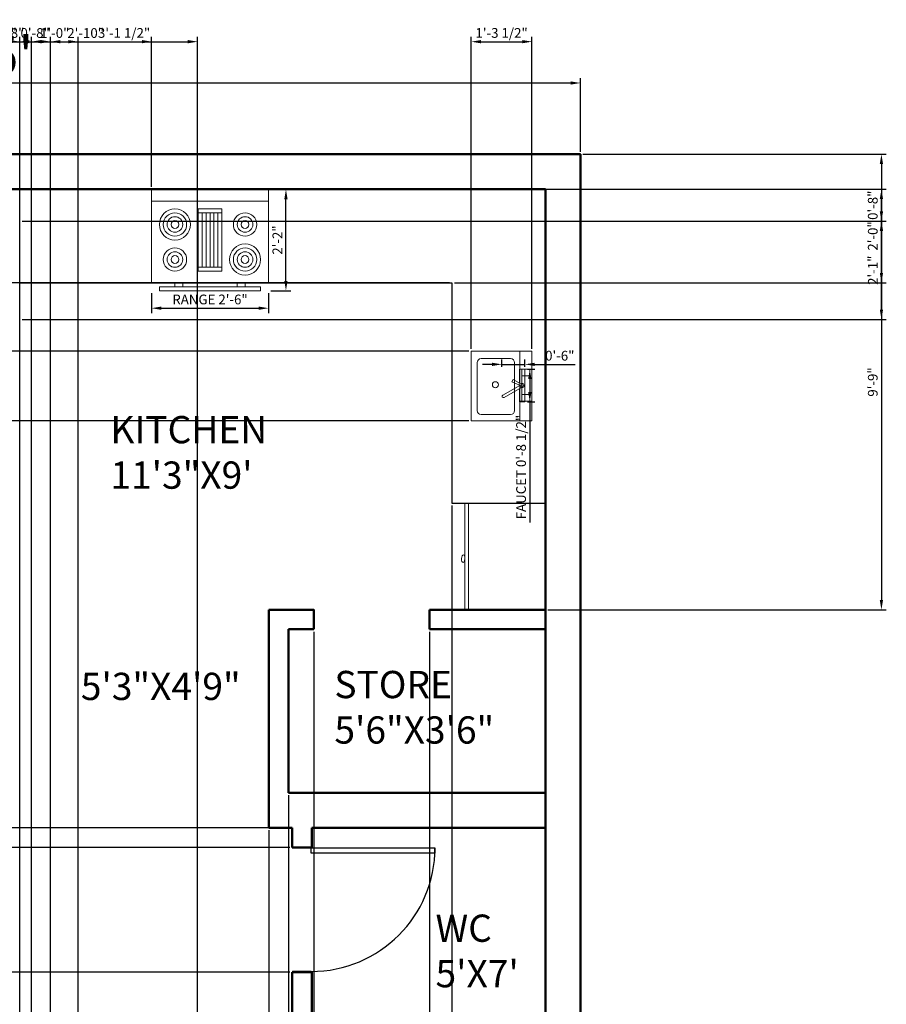
# Model space of a CAD drawing. Units: inches. Extents: x 1854 to 2268, y 1958 to 2535.
# Tile 4 of 4: x 2044 to 2267, y 2283 to 2535. Entities that reach past the tile are written whole.
import ezdxf

# ---------------------------------------------------------------- set-up
doc = ezdxf.new("R2010")
doc.units = ezdxf.units.IN
for name, color, linetype, lineweight in [('A-ANNO-DIMS', 2, 'Continuous', 18), ('A-AREA-IDEN', 7, 'Continuous', 25), ('A-DOOR', 3, 'Continuous', 25), ('A-EQPM', 9, 'Continuous', 18), ('A-FLOR-CASE', 30, 'Continuous', 25), ('A-FLOR-FIXT', 9, 'Continuous', 18), ('A-WALL', 7, 'Continuous', 50)]:
    doc.layers.add(name, color=color, linetype=linetype, lineweight=lineweight)
doc.styles.get("Standard").update_dxf_attribs({"font": 'arial.ttf'})
doc.dimstyles.new('ISO-25', dxfattribs={"dimtxt": 2.5, "dimasz": 2.5, "dimexe": 1.25, "dimexo": 0.625, "dimtad": 1, "dimdec": 0, "dimlunit": 3, "dimtxsty": 'Standard', "dimcen": 2.5, "dimadec": 0, "dimazin": 0, "dimtfac": 1, "dimtdec": 0, "dimtmove": 0, "dimatfit": 3, "dimfxl": 1, "dimarcsym": 0})

# ---------------------------------------------------------------- blocks, each defined once
blk = doc.blocks.new('Range-Oven - 30 in top')
for p, q in [((0, -3), (30, -3)), ((12, -6), (18, -6)), ((13, -20), (13, -6)), ((14, -6), (14, -20)), ((15, -20), (15, -6)), ((16, -6), (16, -20)), ((17, -20), (17, -6)), ((18, -20), (12, -20)), ((6, -24), (6, -25)), ((8, -25), (8, -24)), ((22, -25), (22, -24)), ((24, -24), (24, -25))]:
    blk.add_line(p, q)
for points in [[(0, -24), (0, 0), (30, 0), (30, -24)], [(12, -21), (12, -5), (18, -5), (18, -21)], [(2, -26), (2, -25), (28, -25), (28, -26)]]:
    blk.add_lwpolyline(points, close=True)
for centre, radius in [((6, -9), 4), ((6, -9), 3), ((6, -9), 2), ((24, -9), 3), ((24, -9), 2), ((6, -9), 1), ((24, -9), 1), ((6, -18), 3), ((24, -18), 4), ((24, -18), 3), ((6, -18), 2), ((6, -18), 1), ((24, -18), 2), ((24, -18), 1)]:
    blk.add_circle(centre, radius)
blk = doc.blocks.new('Faucet - single handle top')
for p, q in [((0.08, -0.26), (-2.26, -4.34)), ((-1.37, -4.79), (0.55, -0.5)), ((-0.06, -1.9), (3.57, -8.18)), ((4.43, -7.68), (0.72, -1.24)), ((-2.26, -4.34), (-1.37, -4.79))]:
    blk.add_line(p, q)
for points in [[(-0.92, -2), (-6, -2), (-6, 0), (6, 0), (6, -2), (1.16, -2)], [(-0.01, -2), (-0.12, -2)]]:
    blk.add_lwpolyline(points)
for centre, radius, start, end in [((0, -1), 0.75, 269.2246, 216.2304), ((4, -7.93), 0.5, 210, 30)]:
    blk.add_arc(centre, radius, start, end)
blk = doc.blocks.new('*U13')
for p, q in [((-40, 0), (-40, 6)), ((0, 0), (0, 6))]:
    blk.add_line(p, q)
blk.add_lwpolyline([(0, 0), (0, -40), (-1.75, -40), (-1.75, 0)], close=True)
blk.add_arc((0, 0), 40, 180, 270)
blk = doc.blocks.new('*D16')
at = {"layer": 'A-ANNO-DIMS', "color": 0, "lineweight": -2, "transparency": 16777216}
for p, q in [((1888.43, 2501.46), (1888.43, 2520.38)), ((1890.93, 2519.13), (2185.93, 2519.13)), ((2188.43, 2501.46), (2188.43, 2520.38))]:
    blk.add_line(p, q, dxfattribs=at)
at = {"layer": 'A-ANNO-DIMS', "color": 0, "transparency": 16777216}
for points in [[(1890.93, 2519.54), (1890.93, 2518.71), (1888.43, 2519.13)], [(2185.93, 2519.54), (2185.93, 2518.71), (2188.43, 2519.13)]]:
    blk.add_solid(points, dxfattribs=at)
at = {"layer": 'Defpoints', "color": 0, "transparency": 16777216}
for p in [(2188.43, 2519.13), (1888.43, 2500.84), (2188.43, 2500.84)]:
    blk.add_point(p, dxfattribs=at)
at = {"layer": 'A-ANNO-DIMS', "color": 0, "transparency": 16777216, "insert": (2038.43, 2524.86), "char_height": 10, "attachment_point": 5}
blk.add_mtext("25'", dxfattribs=at)
blk = doc.blocks.new('*D27')
at = {"layer": 'A-ANNO-DIMS', "color": 0, "lineweight": -2, "transparency": 16777216}
for p, q in [((2078.3, 2465.17), (2078.3, 2460.04)), ((2108.3, 2465.17), (2108.3, 2460.04)), ((2080.8, 2461.29), (2105.8, 2461.29))]:
    blk.add_line(p, q, dxfattribs=at)
at = {"layer": 'A-ANNO-DIMS', "color": 0, "transparency": 16777216}
for points in [[(2080.8, 2461.71), (2080.8, 2460.87), (2078.3, 2461.29)], [(2105.8, 2461.71), (2105.8, 2460.87), (2108.3, 2461.29)]]:
    blk.add_solid(points, dxfattribs=at)
at = {"layer": 'Defpoints', "color": 0, "transparency": 16777216}
for p in [(2078.3, 2465.79), (2108.3, 2465.79), (2108.3, 2461.29)]:
    blk.add_point(p, dxfattribs=at)
at = {"layer": 'A-ANNO-DIMS', "color": 0, "transparency": 16777216, "insert": (2093.3, 2463.21), "char_height": 2.5, "attachment_point": 5}
blk.add_mtext('RANGE 2\'-6"', dxfattribs=at)
blk = doc.blocks.new('*D28')
at = {"layer": 'A-ANNO-DIMS', "color": 0, "lineweight": -2, "transparency": 16777216}
for p, q in [((2108.92, 2491.79), (2114.05, 2491.79)), ((2112.8, 2468.29), (2112.8, 2489.29)), ((2108.92, 2465.79), (2114.05, 2465.79))]:
    blk.add_line(p, q, dxfattribs=at)
at = {"layer": 'A-ANNO-DIMS', "color": 0, "transparency": 16777216}
for points in [[(2112.38, 2489.29), (2113.22, 2489.29), (2112.8, 2491.79)], [(2112.38, 2468.29), (2113.22, 2468.29), (2112.8, 2465.79)]]:
    blk.add_solid(points, dxfattribs=at)
at = {"layer": 'Defpoints', "color": 0, "transparency": 16777216}
for p in [(2108.3, 2491.79), (2112.8, 2491.79), (2108.3, 2465.79)]:
    blk.add_point(p, dxfattribs=at)
at = {"layer": 'A-ANNO-DIMS', "color": 0, "transparency": 16777216, "insert": (2110.92, 2478.79), "char_height": 2.5, "attachment_point": 5, "rotation": 90}
blk.add_mtext('2\'-2"', dxfattribs=at)
blk = doc.blocks.new('*D29')
at = {"layer": 'A-ANNO-DIMS', "color": 0, "lineweight": -2, "transparency": 16777216}
for p, q in [((2174.79, 2445.61), (2176.67, 2445.61)), ((2175.42, 2443.11), (2175.42, 2439.76)), ((2174.79, 2437.26), (2176.67, 2437.26)), ((2175.42, 2437.26), (2175.42, 2406.24))]:
    blk.add_line(p, q, dxfattribs=at)
at = {"layer": 'A-ANNO-DIMS', "color": 0, "transparency": 16777216}
for points in [[(2175, 2443.11), (2175.84, 2443.11), (2175.42, 2445.61)], [(2175, 2439.76), (2175.84, 2439.76), (2175.42, 2437.26)]]:
    blk.add_solid(points, dxfattribs=at)
at = {"layer": 'Defpoints', "color": 0, "transparency": 16777216}
for p in [(2174.17, 2445.61), (2174.17, 2437.26), (2175.42, 2437.26)]:
    blk.add_point(p, dxfattribs=at)
at = {"layer": 'A-ANNO-DIMS', "color": 0, "transparency": 16777216, "insert": (2173.5, 2420.5), "char_height": 2.5, "attachment_point": 5, "rotation": 90}
blk.add_mtext('FAUCET 0\'-8 1/2"', dxfattribs=at)
blk = doc.blocks.new('*D30')
at = {"layer": 'A-ANNO-DIMS', "color": 0, "lineweight": -2, "transparency": 16777216}
for p, q in [((2168.25, 2446.24), (2168.25, 2448.12)), ((2174.17, 2446.24), (2174.17, 2448.12)), ((2165.75, 2446.87), (2163.25, 2446.87)), ((2168.25, 2446.87), (2174.17, 2446.87)), ((2176.67, 2446.87), (2187.06, 2446.87))]:
    blk.add_line(p, q, dxfattribs=at)
at = {"layer": 'A-ANNO-DIMS', "color": 0, "transparency": 16777216}
for points in [[(2165.75, 2447.28), (2165.75, 2446.45), (2168.25, 2446.87)], [(2176.67, 2447.28), (2176.67, 2446.45), (2174.17, 2446.87)]]:
    blk.add_solid(points, dxfattribs=at)
at = {"layer": 'Defpoints', "color": 0, "transparency": 16777216}
for p in [(2168.25, 2445.61), (2174.17, 2446.87), (2174.17, 2445.61)]:
    blk.add_point(p, dxfattribs=at)
at = {"layer": 'A-ANNO-DIMS', "color": 0, "transparency": 16777216, "insert": (2183.12, 2448.77), "char_height": 2.5, "attachment_point": 5}
blk.add_mtext('0\'-6"', dxfattribs=at)
blk = doc.blocks.new('*D32')
at = {"layer": 'A-ANNO-DIMS', "color": 0, "lineweight": -2, "transparency": 16777216}
for p, q in [((2035.43, 2492.46), (2035.43, 2530.99)), ((2037.93, 2529.74), (2041.93, 2529.74)), ((2044.43, 2492.46), (2044.43, 2530.99))]:
    blk.add_line(p, q, dxfattribs=at)
at = {"layer": 'A-ANNO-DIMS', "color": 0, "transparency": 16777216}
for points in [[(2037.93, 2530.16), (2037.93, 2529.32), (2035.43, 2529.74)], [(2041.93, 2530.16), (2041.93, 2529.32), (2044.43, 2529.74)]]:
    blk.add_solid(points, dxfattribs=at)
at = {"layer": 'Defpoints', "color": 0, "transparency": 16777216}
for p in [(2044.43, 2529.74), (2035.43, 2491.84), (2044.43, 2491.84)]:
    blk.add_point(p, dxfattribs=at)
at = {"layer": 'A-ANNO-DIMS', "color": 0, "transparency": 16777216, "insert": (2039.93, 2531.64), "char_height": 2.5, "attachment_point": 5}
blk.add_mtext('0\'-9"', dxfattribs=at)
blk = doc.blocks.new('*D36')
at = {"layer": 'A-ANNO-DIMS', "color": 0, "lineweight": -2, "transparency": 16777216}
for p, q in [((2119.96, 2378.21), (2119.96, 1966.69)), ((2149.7, 2378.21), (2149.7, 1966.69)), ((2122.46, 1967.94), (2147.2, 1967.94))]:
    blk.add_line(p, q, dxfattribs=at)
at = {"layer": 'A-ANNO-DIMS', "color": 0, "transparency": 16777216}
for points in [[(2122.46, 1968.36), (2122.46, 1967.52), (2119.96, 1967.94)], [(2147.2, 1968.36), (2147.2, 1967.52), (2149.7, 1967.94)]]:
    blk.add_solid(points, dxfattribs=at)
at = {"layer": 'Defpoints', "color": 0, "transparency": 16777216}
for p in [(2119.96, 2378.84), (2149.7, 2378.84), (2149.7, 1967.94)]:
    blk.add_point(p, dxfattribs=at)
at = {"layer": 'A-ANNO-DIMS', "color": 0, "transparency": 16777216, "insert": (2134.83, 1969.86), "char_height": 2.5, "attachment_point": 5}
blk.add_mtext('2\'-5 1/2"', dxfattribs=at)
blk = doc.blocks.new('*D37')
at = {"layer": 'A-ANNO-DIMS', "color": 0, "lineweight": -2, "transparency": 16777216}
for p, q in [((2113.81, 2322.77), (1858.28, 2322.77)), ((1859.53, 2320.27), (1859.53, 2293.27)), ((2113.81, 2290.77), (1858.28, 2290.77))]:
    blk.add_line(p, q, dxfattribs=at)
at = {"layer": 'A-ANNO-DIMS', "color": 0, "transparency": 16777216}
for points in [[(1859.12, 2320.27), (1859.95, 2320.27), (1859.53, 2322.77)], [(1859.12, 2293.27), (1859.95, 2293.27), (1859.53, 2290.77)]]:
    blk.add_solid(points, dxfattribs=at)
at = {"layer": 'Defpoints', "color": 0, "transparency": 16777216}
for p in [(2114.43, 2322.77), (1859.53, 2290.77), (2114.43, 2290.77)]:
    blk.add_point(p, dxfattribs=at)
at = {"layer": 'A-ANNO-DIMS', "color": 0, "transparency": 16777216, "insert": (1857.63, 2306.77), "char_height": 2.5, "attachment_point": 5, "rotation": 90}
blk.add_mtext('2\'-8"', dxfattribs=at)
blk = doc.blocks.new('*D43')
at = {"layer": 'A-ANNO-DIMS', "color": 0, "lineweight": -2, "transparency": 16777216}
for p, q in [((2052.36, 2115.46), (2052.36, 2530.99)), ((2054.86, 2529.74), (2087.6, 2529.74)), ((2090.1, 2115.46), (2090.1, 2530.99))]:
    blk.add_line(p, q, dxfattribs=at)
at = {"layer": 'A-ANNO-DIMS', "color": 0, "transparency": 16777216}
for points in [[(2054.86, 2530.16), (2054.86, 2529.32), (2052.36, 2529.74)], [(2087.6, 2530.16), (2087.6, 2529.32), (2090.1, 2529.74)]]:
    blk.add_solid(points, dxfattribs=at)
at = {"layer": 'Defpoints', "color": 0, "transparency": 16777216}
for p in [(2090.1, 2529.74), (2052.36, 2114.84), (2090.1, 2114.84)]:
    blk.add_point(p, dxfattribs=at)
at = {"layer": 'A-ANNO-DIMS', "color": 0, "transparency": 16777216, "insert": (2071.23, 2531.66), "char_height": 2.5, "attachment_point": 5}
blk.add_mtext('3\'-1 1/2"', dxfattribs=at)
blk = doc.blocks.new('*D44')
at = {"layer": 'A-ANNO-DIMS', "color": 0, "lineweight": -2, "transparency": 16777216}
for p, q in [((2045.06, 2483.65), (2266.96, 2483.65)), ((2265.71, 2460.93), (2265.71, 2481.15)), ((2045.06, 2458.43), (2266.96, 2458.43))]:
    blk.add_line(p, q, dxfattribs=at)
at = {"layer": 'A-ANNO-DIMS', "color": 0, "transparency": 16777216}
for points in [[(2265.29, 2481.15), (2266.13, 2481.15), (2265.71, 2483.65)], [(2265.29, 2460.93), (2266.13, 2460.93), (2265.71, 2458.43)]]:
    blk.add_solid(points, dxfattribs=at)
at = {"layer": 'Defpoints', "color": 0, "transparency": 16777216}
for p in [(2044.43, 2483.65), (2265.71, 2483.65), (2044.43, 2458.43)]:
    blk.add_point(p, dxfattribs=at)
at = {"layer": 'A-ANNO-DIMS', "color": 0, "transparency": 16777216, "insert": (2263.83, 2471.04), "char_height": 2.5, "attachment_point": 5, "rotation": 90}
blk.add_mtext('2\'-1"', dxfattribs=at)
blk = doc.blocks.new('*D51')
at = {"layer": 'A-ANNO-DIMS', "color": 0, "lineweight": -2, "transparency": 16777216}
for p, q in [((2027.6, 2450.46), (2027.6, 2530.99)), ((2030.1, 2529.74), (2032.93, 2529.74)), ((2035.43, 2450.46), (2035.43, 2530.99)), ((2035.43, 2529.74), (2045.83, 2529.74))]:
    blk.add_line(p, q, dxfattribs=at)
at = {"layer": 'A-ANNO-DIMS', "color": 0, "transparency": 16777216}
for points in [[(2030.1, 2530.16), (2030.1, 2529.32), (2027.6, 2529.74)], [(2032.93, 2530.16), (2032.93, 2529.32), (2035.43, 2529.74)]]:
    blk.add_solid(points, dxfattribs=at)
at = {"layer": 'Defpoints', "color": 0, "transparency": 16777216}
for p in [(2035.43, 2529.74), (2027.6, 2449.84), (2035.43, 2449.84)]:
    blk.add_point(p, dxfattribs=at)
at = {"layer": 'A-ANNO-DIMS', "color": 0, "transparency": 16777216, "insert": (2041.88, 2531.64), "char_height": 2.5, "attachment_point": 5}
blk.add_mtext('0\'-8"', dxfattribs=at)
blk = doc.blocks.new('*D52')
at = {"layer": 'A-ANNO-DIMS', "color": 0, "lineweight": -2, "transparency": 16777216}
for p, q in [((2149.7, 2378.21), (2149.7, 1966.69)), ((2179.43, 2378.21), (2179.43, 1966.69)), ((2152.2, 1967.94), (2176.93, 1967.94))]:
    blk.add_line(p, q, dxfattribs=at)
at = {"layer": 'A-ANNO-DIMS', "color": 0, "transparency": 16777216}
for points in [[(2152.2, 1968.36), (2152.2, 1967.52), (2149.7, 1967.94)], [(2176.93, 1968.36), (2176.93, 1967.52), (2179.43, 1967.94)]]:
    blk.add_solid(points, dxfattribs=at)
at = {"layer": 'Defpoints', "color": 0, "transparency": 16777216}
for p in [(2149.7, 2378.84), (2179.43, 2378.84), (2179.43, 1967.94)]:
    blk.add_point(p, dxfattribs=at)
at = {"layer": 'A-ANNO-DIMS', "color": 0, "transparency": 16777216, "insert": (2164.57, 1969.86), "char_height": 2.5, "attachment_point": 5}
blk.add_mtext('2\'-5 1/2"', dxfattribs=at)
blk = doc.blocks.new('*D53')
at = {"layer": 'A-ANNO-DIMS', "color": 0, "lineweight": -2, "transparency": 16777216}
for p, q in [((2189.06, 2500.84), (2266.96, 2500.84)), ((2265.71, 2498.34), (2265.71, 2386.34)), ((2180.06, 2383.84), (2266.96, 2383.84))]:
    blk.add_line(p, q, dxfattribs=at)
at = {"layer": 'A-ANNO-DIMS', "color": 0, "transparency": 16777216}
for points in [[(2265.29, 2498.34), (2266.13, 2498.34), (2265.71, 2500.84)], [(2265.29, 2386.34), (2266.13, 2386.34), (2265.71, 2383.84)]]:
    blk.add_solid(points, dxfattribs=at)
at = {"layer": 'Defpoints', "color": 0, "transparency": 16777216}
for p in [(2188.43, 2500.84), (2179.43, 2383.84), (2265.71, 2383.84)]:
    blk.add_point(p, dxfattribs=at)
at = {"layer": 'A-ANNO-DIMS', "color": 0, "transparency": 16777216, "insert": (2263.81, 2442.34), "char_height": 2.5, "attachment_point": 5, "rotation": 90}
blk.add_mtext('9\'-9"', dxfattribs=at)
blk = doc.blocks.new('*D55')
at = {"layer": 'A-ANNO-DIMS', "color": 0, "lineweight": -2, "transparency": 16777216}
for p, q in [((2044.43, 2492.46), (2044.43, 2530.99)), ((2046.93, 2529.74), (2075.8, 2529.74)), ((2078.3, 2492.42), (2078.3, 2530.99))]:
    blk.add_line(p, q, dxfattribs=at)
at = {"layer": 'A-ANNO-DIMS', "color": 0, "transparency": 16777216}
for points in [[(2046.93, 2530.16), (2046.93, 2529.32), (2044.43, 2529.74)], [(2075.8, 2530.16), (2075.8, 2529.32), (2078.3, 2529.74)]]:
    blk.add_solid(points, dxfattribs=at)
at = {"layer": 'Defpoints', "color": 0, "transparency": 16777216}
for p in [(2078.3, 2529.74), (2044.43, 2491.84), (2078.3, 2491.79)]:
    blk.add_point(p, dxfattribs=at)
at = {"layer": 'A-ANNO-DIMS', "color": 0, "transparency": 16777216, "insert": (2061.37, 2531.64), "char_height": 2.5, "attachment_point": 5}
blk.add_mtext('2\'-10"', dxfattribs=at)
blk = doc.blocks.new('*D56')
at = {"layer": 'A-ANNO-DIMS', "color": 0, "lineweight": -2, "transparency": 16777216}
for p, q in [((2155.43, 2410.58), (2155.43, 1966.69)), ((2179.43, 2410.58), (2179.43, 1966.69)), ((2157.93, 1967.94), (2176.93, 1967.94))]:
    blk.add_line(p, q, dxfattribs=at)
at = {"layer": 'A-ANNO-DIMS', "color": 0, "transparency": 16777216}
for points in [[(2157.93, 1968.36), (2157.93, 1967.52), (2155.43, 1967.94)], [(2176.93, 1968.36), (2176.93, 1967.52), (2179.43, 1967.94)]]:
    blk.add_solid(points, dxfattribs=at)
at = {"layer": 'Defpoints', "color": 0, "transparency": 16777216}
for p in [(2155.43, 2411.2), (2179.43, 2411.2), (2179.43, 1967.94)]:
    blk.add_point(p, dxfattribs=at)
at = {"layer": 'A-ANNO-DIMS', "color": 0, "transparency": 16777216, "insert": (2167.43, 1969.84), "char_height": 2.5, "attachment_point": 5}
blk.add_mtext('2\'-0"', dxfattribs=at)
blk = doc.blocks.new('*D57')
at = {"layer": 'A-ANNO-DIMS', "color": 0, "lineweight": -2, "transparency": 16777216}
for p, q in [((2180.06, 2491.84), (2266.96, 2491.84)), ((2265.71, 2470.34), (2265.71, 2489.34)), ((2156.06, 2467.84), (2266.96, 2467.84))]:
    blk.add_line(p, q, dxfattribs=at)
at = {"layer": 'A-ANNO-DIMS', "color": 0, "transparency": 16777216}
for points in [[(2265.29, 2489.34), (2266.13, 2489.34), (2265.71, 2491.84)], [(2265.29, 2470.34), (2266.13, 2470.34), (2265.71, 2467.84)]]:
    blk.add_solid(points, dxfattribs=at)
at = {"layer": 'Defpoints', "color": 0, "transparency": 16777216}
for p in [(2179.43, 2491.84), (2265.71, 2491.84), (2155.43, 2467.84)]:
    blk.add_point(p, dxfattribs=at)
at = {"layer": 'A-ANNO-DIMS', "color": 0, "transparency": 16777216, "insert": (2263.81, 2479.84), "char_height": 2.5, "attachment_point": 5, "rotation": 90}
blk.add_mtext('2\'-0"', dxfattribs=at)
blk = doc.blocks.new('*D65')
at = {"layer": 'A-ANNO-DIMS', "color": 0, "lineweight": -2, "transparency": 16777216}
for p, q in [((2047.43, 2106.33), (2047.43, 2530.99)), ((2049.93, 2529.74), (2056.93, 2529.74)), ((2059.43, 2106.33), (2059.43, 2530.99))]:
    blk.add_line(p, q, dxfattribs=at)
at = {"layer": 'A-ANNO-DIMS', "color": 0, "transparency": 16777216}
for points in [[(2049.93, 2530.16), (2049.93, 2529.32), (2047.43, 2529.74)], [(2056.93, 2530.16), (2056.93, 2529.32), (2059.43, 2529.74)]]:
    blk.add_solid(points, dxfattribs=at)
at = {"layer": 'Defpoints', "color": 0, "transparency": 16777216}
for p in [(2059.43, 2529.74), (2047.43, 2105.7), (2059.43, 2105.7)]:
    blk.add_point(p, dxfattribs=at)
at = {"layer": 'A-ANNO-DIMS', "color": 0, "transparency": 16777216, "insert": (2053.43, 2531.64), "char_height": 2.5, "attachment_point": 5}
blk.add_mtext('1\'-0"', dxfattribs=at)
blk = doc.blocks.new('*D66')
at = {"layer": 'A-ANNO-DIMS', "color": 0, "lineweight": -2, "transparency": 16777216}
for p, q in [((2044.43, 2115.46), (2044.43, 2530.99)), ((2046.93, 2529.74), (2049.86, 2529.74)), ((2052.36, 2115.46), (2052.36, 2530.99))]:
    blk.add_line(p, q, dxfattribs=at)
at = {"layer": 'A-ANNO-DIMS', "color": 0, "transparency": 16777216}
for points in [[(2046.93, 2530.16), (2046.93, 2529.32), (2044.43, 2529.74)], [(2049.86, 2530.16), (2049.86, 2529.32), (2052.36, 2529.74)]]:
    blk.add_solid(points, dxfattribs=at)
at = {"layer": 'Defpoints', "color": 0, "transparency": 16777216}
for p in [(2052.36, 2529.74), (2044.43, 2114.84), (2052.36, 2114.84)]:
    blk.add_point(p, dxfattribs=at)
at = {"layer": 'A-ANNO-DIMS', "color": 0, "transparency": 16777216, "insert": (2048.4, 2531.64), "char_height": 2.5, "attachment_point": 5}
blk.add_mtext('0\'-8"', dxfattribs=at)
blk = doc.blocks.new('*D70')
at = {"layer": 'A-ANNO-DIMS', "color": 0, "lineweight": -2, "transparency": 16777216}
for p, q in [((1859.53, 2330.34), (1859.53, 2340.74)), ((2113.81, 2327.84), (1858.28, 2327.84)), ((1859.53, 2322.77), (1859.53, 2327.84)), ((2113.81, 2322.77), (1858.28, 2322.77)), ((1859.53, 2320.27), (1859.53, 2317.77))]:
    blk.add_line(p, q, dxfattribs=at)
at = {"layer": 'A-ANNO-DIMS', "color": 0, "transparency": 16777216}
for points in [[(1859.12, 2330.34), (1859.95, 2330.34), (1859.53, 2327.84)], [(1859.12, 2320.27), (1859.95, 2320.27), (1859.53, 2322.77)]]:
    blk.add_solid(points, dxfattribs=at)
at = {"layer": 'Defpoints', "color": 0, "transparency": 16777216}
for p in [(1859.53, 2327.84), (2114.43, 2327.84), (2114.43, 2322.77)]:
    blk.add_point(p, dxfattribs=at)
at = {"layer": 'A-ANNO-DIMS', "color": 0, "transparency": 16777216, "insert": (1857.63, 2336.79), "char_height": 2.5, "attachment_point": 5, "rotation": 90}
blk.add_mtext('0\'-5"', dxfattribs=at)
blk = doc.blocks.new('*D71')
at = {"layer": 'A-ANNO-DIMS', "color": 0, "lineweight": -2, "transparency": 16777216}
for p, q in [((2045.06, 2491.84), (2266.96, 2491.84)), ((2265.71, 2489.34), (2265.71, 2486.15)), ((2045.06, 2483.65), (2266.96, 2483.65))]:
    blk.add_line(p, q, dxfattribs=at)
at = {"layer": 'A-ANNO-DIMS', "color": 0, "transparency": 16777216}
for points in [[(2265.29, 2489.34), (2266.13, 2489.34), (2265.71, 2491.84)], [(2265.29, 2486.15), (2266.13, 2486.15), (2265.71, 2483.65)]]:
    blk.add_solid(points, dxfattribs=at)
at = {"layer": 'Defpoints', "color": 0, "transparency": 16777216}
for p in [(2044.43, 2491.84), (2044.43, 2483.65), (2265.71, 2483.65)]:
    blk.add_point(p, dxfattribs=at)
at = {"layer": 'A-ANNO-DIMS', "color": 0, "transparency": 16777216, "insert": (2263.81, 2487.74), "char_height": 2.5, "attachment_point": 5, "rotation": 90}
blk.add_mtext('0\'-8"', dxfattribs=at)
blk = doc.blocks.new('*D72')
at = {"layer": 'A-ANNO-DIMS', "color": 0, "lineweight": -2, "transparency": 16777216}
for p, q in [((2160.38, 2450.89), (2160.38, 2530.99)), ((2162.88, 2529.74), (2173.48, 2529.74)), ((2175.98, 2450.89), (2175.98, 2530.99))]:
    blk.add_line(p, q, dxfattribs=at)
at = {"layer": 'A-ANNO-DIMS', "color": 0, "transparency": 16777216}
for points in [[(2162.88, 2530.16), (2162.88, 2529.32), (2160.38, 2529.74)], [(2173.48, 2530.16), (2173.48, 2529.32), (2175.98, 2529.74)]]:
    blk.add_solid(points, dxfattribs=at)
at = {"layer": 'Defpoints', "color": 0, "transparency": 16777216}
for p in [(2175.98, 2529.74), (2160.38, 2450.27), (2175.98, 2450.27)]:
    blk.add_point(p, dxfattribs=at)
at = {"layer": 'A-ANNO-DIMS', "color": 0, "transparency": 16777216, "insert": (2168.18, 2531.66), "char_height": 2.5, "attachment_point": 5}
blk.add_mtext('1\'-3 1/2"', dxfattribs=at)
blk = doc.blocks.new('*D73')
at = {"layer": 'A-ANNO-DIMS', "color": 0, "lineweight": -2, "transparency": 16777216}
for p, q in [((2159.76, 2450.27), (1858.28, 2450.27)), ((1859.53, 2434.83), (1859.53, 2447.77)), ((2159.76, 2432.33), (1858.28, 2432.33))]:
    blk.add_line(p, q, dxfattribs=at)
at = {"layer": 'A-ANNO-DIMS', "color": 0, "transparency": 16777216}
for points in [[(1859.12, 2447.77), (1859.95, 2447.77), (1859.53, 2450.27)], [(1859.12, 2434.83), (1859.95, 2434.83), (1859.53, 2432.33)]]:
    blk.add_solid(points, dxfattribs=at)
at = {"layer": 'Defpoints', "color": 0, "transparency": 16777216}
for p in [(1859.53, 2450.27), (2160.38, 2450.27), (2160.38, 2432.33)]:
    blk.add_point(p, dxfattribs=at)
at = {"layer": 'A-ANNO-DIMS', "color": 0, "transparency": 16777216, "insert": (1857.63, 2441.3), "char_height": 2.5, "attachment_point": 5, "rotation": 90}
blk.add_mtext('1\'-6"', dxfattribs=at)
blk = doc.blocks.new('*D74')
at = {"layer": 'A-ANNO-DIMS', "color": 0, "lineweight": -2, "transparency": 16777216}
for p, q in [((2154.81, 2467.84), (1858.28, 2467.84)), ((1859.53, 2452.77), (1859.53, 2465.34)), ((2159.76, 2450.27), (1858.28, 2450.27))]:
    blk.add_line(p, q, dxfattribs=at)
at = {"layer": 'A-ANNO-DIMS', "color": 0, "transparency": 16777216}
for points in [[(1859.12, 2465.34), (1859.95, 2465.34), (1859.53, 2467.84)], [(1859.12, 2452.77), (1859.95, 2452.77), (1859.53, 2450.27)]]:
    blk.add_solid(points, dxfattribs=at)
at = {"layer": 'Defpoints', "color": 0, "transparency": 16777216}
for p in [(1859.53, 2467.84), (2155.43, 2467.84), (2160.38, 2450.27)]:
    blk.add_point(p, dxfattribs=at)
at = {"layer": 'A-ANNO-DIMS', "color": 0, "transparency": 16777216, "insert": (1857.61, 2459.05), "char_height": 2.5, "attachment_point": 5, "rotation": 90}
blk.add_mtext('1\'-5 1/2"', dxfattribs=at)
blk = doc.blocks.new('*D79')
at = {"layer": 'A-ANNO-DIMS', "color": 0, "lineweight": -2, "transparency": 16777216}
for p, q in [((2113.43, 2336.21), (2113.43, 1966.69)), ((2108.43, 2327.21), (2108.43, 1966.69)), ((2105.93, 1967.94), (2103.43, 1967.94)), ((2108.43, 1967.94), (2113.43, 1967.94)), ((2115.93, 1967.94), (2126.33, 1967.94))]:
    blk.add_line(p, q, dxfattribs=at)
at = {"layer": 'A-ANNO-DIMS', "color": 0, "transparency": 16777216}
for points in [[(2105.93, 1968.36), (2105.93, 1967.52), (2108.43, 1967.94)], [(2115.93, 1968.36), (2115.93, 1967.52), (2113.43, 1967.94)]]:
    blk.add_solid(points, dxfattribs=at)
at = {"layer": 'Defpoints', "color": 0, "transparency": 16777216}
for p in [(2113.43, 2336.84), (2108.43, 2327.84), (2113.43, 1967.94)]:
    blk.add_point(p, dxfattribs=at)
at = {"layer": 'A-ANNO-DIMS', "color": 0, "transparency": 16777216, "insert": (2122.38, 1969.84), "char_height": 2.5, "attachment_point": 5}
blk.add_mtext('0\'-5"', dxfattribs=at)

msp = doc.modelspace()

# ---------------------------------------------------------------- linework, layer by layer
at = {"layer": 'A-EQPM'}
for p, q in [((2158.72, 2411.2), (2158.72, 2383.84)), ((2159.65, 2383.84), (2159.65, 2411.2)), ((2163.97, 2383.84), (2164.57, 2383.84))]:
    msp.add_line(p, q, dxfattribs=at)
msp.add_ellipse((2158.32, 2396.96), major_axis=(-0.044, -0.999), ratio=0.41834, dxfattribs=at)
at = {"layer": 'A-FLOR-CASE'}
for p, q in [((2044.43, 2467.84), (2155.43, 2467.84)), ((2155.43, 2467.84), (2155.43, 2411.2)), ((2155.43, 2411.2), (2179.43, 2411.2))]:
    msp.add_line(p, q, dxfattribs=at)
at = {"layer": 'A-FLOR-FIXT'}
for p, q in [((2162.91, 2448.34), (2170.49, 2448.34)), ((2172.9, 2450.27), (2172.9, 2432.33)), ((2161.91, 2434.99), (2161.91, 2447.34)), ((2171.49, 2447.34), (2171.49, 2434.99)), ((2172.9, 2445.67), (2175.98, 2445.67)), ((2173.37, 2445.67), (2173.37, 2437.44)), ((2175.42, 2445.67), (2175.42, 2437.44)), ((2173.37, 2443.94), (2175.42, 2443.94)), ((2173.37, 2439.13), (2175.42, 2439.13)), ((2172.9, 2437.44), (2175.98, 2437.44)), ((2170.49, 2433.99), (2162.91, 2433.99))]:
    msp.add_line(p, q, dxfattribs=at)
msp.add_lwpolyline([(2160.38, 2450.27), (2175.98, 2450.27), (2175.98, 2432.33), (2160.38, 2432.33)], close=True, dxfattribs=at)
msp.add_circle((2166.6, 2441.63), 0.786, dxfattribs=at)
for centre, start, end in [((2162.91, 2447.34), 90, 180), ((2170.49, 2447.34), 0, 90), ((2162.91, 2434.99), 180, 270), ((2170.49, 2434.99), 270, 0)]:
    msp.add_arc(centre, 1, start, end, dxfattribs=at)
at = {"layer": 'A-WALL'}
for p, q in [((1897.43, 2491.84), (2179.43, 2491.84)), ((2179.43, 2491.84), (2179.43, 2029.84)), ((2108.43, 2383.84), (2119.96, 2383.84)), ((2108.43, 2383.84), (2108.43, 2327.84)), ((2119.96, 2383.88), (2119.96, 2378.84)), ((2149.7, 2381.4), (2149.7, 2383.84)), ((2149.7, 2383.84), (2149.7, 2378.84)), ((2149.7, 2383.84), (2179.43, 2383.84)), ((2113.43, 2378.84), (2113.43, 2336.84)), ((2113.43, 2378.84), (2119.96, 2378.84)), ((2149.7, 2378.84), (2179.43, 2378.84)), ((2113.43, 2336.84), (2179.43, 2336.84)), ((2108.43, 2327.84), (2114.43, 2327.84)), ((2114.43, 2327.84), (2114.43, 2322.77)), ((2119.43, 2327.84), (2119.43, 2322.77)), ((2119.43, 2327.84), (2179.43, 2327.84)), ((2114.43, 2322.77), (2119.43, 2322.77)), ((2116.93, 2290.77), (2114.43, 2290.77)), ((2114.43, 2290.77), (2119.43, 2290.77)), ((2114.43, 2290.77), (2114.43, 2243.84)), ((2119.43, 2290.77), (2119.43, 2243.84))]:
    msp.add_line(p, q, dxfattribs=at)
msp.add_lwpolyline([(1888.43, 2500.84), (2188.43, 2500.84), (2188.43, 2020.84), (1888.43, 2020.84)], close=True, dxfattribs=at)

# ---------------------------------------------------------------- block references
at = {"layer": 'A-DOOR', "xscale": 0.7945589696422604, "yscale": 0.7945589696422604, "zscale": 0.7945589696422604, "rotation": 90.00000000000003}
msp.add_blockref('*U13', (2119.29, 2322.74), dxfattribs=at)
at = {"layer": 'A-EQPM'}
msp.add_blockref('Range-Oven - 30 in top', (2078.3, 2491.79), dxfattribs=at)
at = {"layer": 'A-FLOR-FIXT', "xscale": 0.6959038539063253, "yscale": 0.6959038539063253, "zscale": 0.6959038539063253, "rotation": 270}
msp.add_blockref('Faucet - single handle top', (2174.17, 2441.44), dxfattribs=at)

# ---------------------------------------------------------------- texts
at = {"layer": 'A-AREA-IDEN', "char_height": 7, "attachment_point": 1}
for s, insert in [('KITCHEN\\P11\'3"X9\'', (2067.72, 2433.6)), ('5\'3"X4\'9"', (2060.13, 2367.67)), ('STORE\\P5\'6"X3\'6"', (2125.24, 2368.14)), ("WC\\P5'X7'", (2151.21, 2305.56))]:
    msp.add_mtext_dynamic_manual_height_columns(s, width=76.0498, gutter_width=12.5, heights=[0], dxfattribs=dict(at, insert=insert))

# ---------------------------------------------------------------- dimensions: what is measured, and where the dimension line sits
at = {"layer": 'A-ANNO-DIMS'}
for base, p1, p2, override, picture, middle in [((2090.1, 2529.74), (2052.36, 2114.84), (2090.1, 2114.84), {"dimdec": 1, "dimlfac": 1, "dimrnd": 0, "dimzin": 1, "dimdsep": 46, "dimlunit": 4, "dimfrac": 2}, '*D43', (2071.23, 2531.66)), ((2175.98, 2529.74), (2160.38, 2450.27), (2175.98, 2450.27), {"dimdec": 1, "dimlfac": 1, "dimrnd": 0, "dimzin": 1, "dimdsep": 46, "dimlunit": 4, "dimfrac": 2}, '*D72', (2168.18, 2531.66)), ((2188.43, 2519.13), (1888.43, 2500.84), (2188.43, 2500.84), {"dimtxt": 10, "dimclrd": 0, "dimclre": 0, "dimclrt": 0}, '*D16', (2038.43, 2524.86)), ((2035.43, 2529.74), (2027.6, 2449.84), (2035.43, 2449.84), {"dimdec": 1, "dimlfac": 1, "dimrnd": 0, "dimzin": 1, "dimdsep": 46, "dimlunit": 4, "dimfrac": 2}, '*D51', (2041.88, 2531.64)), ((2044.43, 2529.74), (2035.43, 2491.84), (2044.43, 2491.84), {"dimdec": 1, "dimlfac": 1, "dimrnd": 0, "dimzin": 1, "dimdsep": 46, "dimlunit": 4, "dimfrac": 2}, '*D32', (2039.93, 2531.64)), ((2078.3, 2529.74), (2044.43, 2491.84), (2078.3, 2491.79), {"dimdec": 1, "dimlfac": 1, "dimrnd": 0, "dimzin": 1, "dimdsep": 46, "dimlunit": 4, "dimfrac": 2}, '*D55', (2061.37, 2531.64)), ((2052.36, 2529.74), (2044.43, 2114.84), (2052.36, 2114.84), {"dimdec": 1, "dimlfac": 1, "dimrnd": 0, "dimzin": 1, "dimdsep": 46, "dimlunit": 4, "dimfrac": 2}, '*D66', (2048.4, 2531.64)), ((2059.43, 2529.74), (2047.43, 2105.7), (2059.43, 2105.7), {"dimdec": 1, "dimlfac": 1, "dimrnd": 0, "dimzin": 1, "dimdsep": 46, "dimlunit": 4, "dimfrac": 2}, '*D65', (2053.43, 2531.64)), ((2174.17, 2446.87), (2168.25, 2445.61), (2174.17, 2445.61), {"dimdec": 1, "dimlfac": 1, "dimrnd": 0, "dimzin": 1, "dimdsep": 46, "dimlunit": 4, "dimfrac": 2}, '*D30', (2183.12, 2448.77)), ((2179.43, 1967.94), (2155.43, 2411.2), (2179.43, 2411.2), {"dimdec": 1, "dimlfac": 1, "dimrnd": 0, "dimzin": 1, "dimdsep": 46, "dimlunit": 4, "dimfrac": 2}, '*D56', (2167.43, 1969.84)), ((2149.7, 1967.94), (2119.96, 2378.84), (2149.7, 2378.84), {"dimdec": 1, "dimlfac": 1, "dimrnd": 0, "dimzin": 1, "dimdsep": 46, "dimlunit": 4, "dimfrac": 2}, '*D36', (2134.83, 1969.86)), ((2179.43, 1967.94), (2149.7, 2378.84), (2179.43, 2378.84), {"dimdec": 1, "dimlfac": 1, "dimrnd": 0, "dimzin": 1, "dimdsep": 46, "dimlunit": 4, "dimfrac": 2}, '*D52', (2164.57, 1969.86)), ((2113.43, 1967.94), (2108.43, 2327.84), (2113.43, 2336.84), {"dimdec": 1, "dimlfac": 1, "dimrnd": 0, "dimzin": 1, "dimdsep": 46, "dimlunit": 4, "dimfrac": 2}, '*D79', (2122.38, 1969.84))]:
    dim = msp.add_linear_dim(base=base, p1=p1, p2=p2, dimstyle='ISO-25', override=override, dxfattribs=at)
    dim.commit()
    dim.dimension.update_dxf_attribs({"geometry": picture, "text_midpoint": middle})
for base, p1, p2, picture, middle in [((2265.71, 2383.84), (2188.43, 2500.84), (2179.43, 2383.84), '*D53', (2263.81, 2442.34)), ((2265.71, 2483.65), (2044.43, 2491.84), (2044.43, 2483.65), '*D71', (2263.81, 2487.74)), ((2112.8, 2491.79), (2108.3, 2465.79), (2108.3, 2491.79), '*D28', (2110.92, 2478.79)), ((2265.71, 2491.84), (2155.43, 2467.84), (2179.43, 2491.84), '*D57', (2263.81, 2479.84)), ((2265.71, 2483.65), (2044.43, 2458.43), (2044.43, 2483.65), '*D44', (2263.83, 2471.04)), ((1859.53, 2467.84), (2160.38, 2450.27), (2155.43, 2467.84), '*D74', (1857.61, 2459.05)), ((1859.53, 2450.27), (2160.38, 2432.33), (2160.38, 2450.27), '*D73', (1857.63, 2441.3)), ((1859.53, 2327.84), (2114.43, 2322.77), (2114.43, 2327.84), '*D70', (1857.63, 2336.79)), ((1859.53, 2290.77), (2114.43, 2322.77), (2114.43, 2290.77), '*D37', (1857.63, 2306.77))]:
    dim = msp.add_linear_dim(base=base, p1=p1, p2=p2, angle=90, dimstyle='ISO-25', override={"dimdec": 1, "dimlfac": 1, "dimrnd": 0, "dimzin": 1, "dimdsep": 46, "dimlunit": 4, "dimfrac": 2}, dxfattribs=at)
    dim.commit()
    dim.dimension.update_dxf_attribs({"geometry": picture, "text_midpoint": middle})
dim = msp.add_linear_dim(base=(2108.3, 2461.29), p1=(2078.3, 2465.79), p2=(2108.3, 2465.79), text='RANGE <>', dimstyle='ISO-25', override={"dimdec": 1, "dimlfac": 1, "dimrnd": 0, "dimzin": 1, "dimdsep": 46, "dimlunit": 4, "dimfrac": 2}, dxfattribs=at)
dim.commit()
dim.dimension.update_dxf_attribs({"geometry": '*D27', "text_midpoint": (2093.3, 2463.21)})
dim = msp.add_linear_dim(base=(2175.4208, 2437.2638), p1=(2174.1682, 2445.6146), p2=(2174.1682, 2437.2638), angle=270, text='FAUCET <>', dimstyle='ISO-25', override={"dimdec": 1, "dimlfac": 1, "dimrnd": 0, "dimzin": 1, "dimdsep": 46, "dimlunit": 4, "dimfrac": 2}, dxfattribs=at)
dim.commit()
dim.dimension.update_dxf_attribs({"geometry": '*D29', "text_midpoint": (2173.5031, 2420.5039)})

doc.saveas('drawing.dxf')
